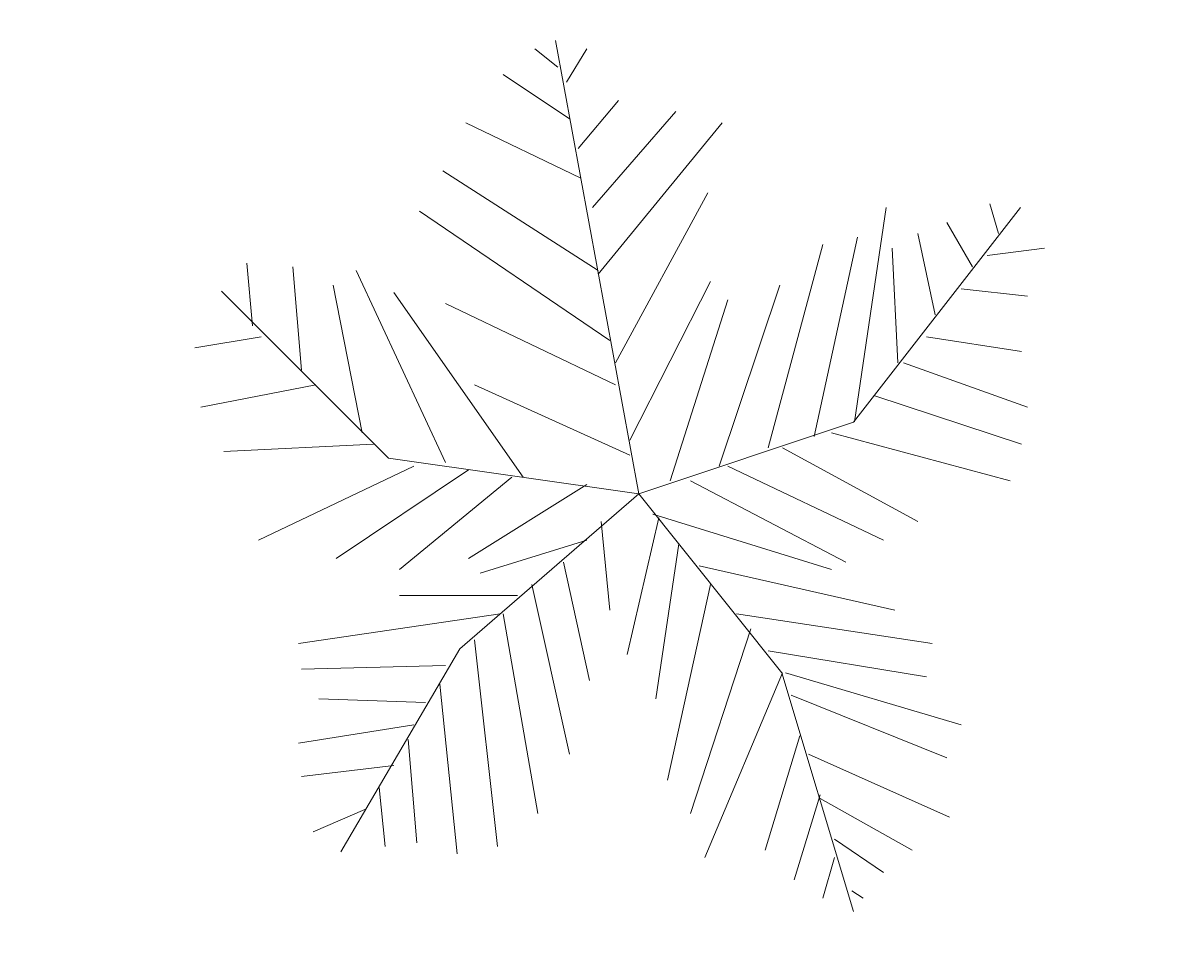
# Model space of a CAD drawing. Units: inches. Extents: x -61 to 1599, y -1316 to 257.
# Tile 127 of 204: x 388 to 418, y -166 to -143. Entities that reach past the tile are written whole.
import ezdxf

# ---------------------------------------------------------------- set-up
doc = ezdxf.new("R2010")
doc.units = ezdxf.units.IN
doc.header["$MEASUREMENT"] = 0
doc.layers.add('A-ANNO-DIMS', color=2, linetype='Continuous', lineweight=18)
doc.layers.add('FURNITURE', color=83, linetype='Continuous', lineweight=18)
doc.styles.get("Standard").update_dxf_attribs({"font": 'arial.ttf'})
doc.dimstyles.get("Standard").update_dxf_attribs({"dimtxt": 0.18, "dimasz": 0.18, "dimexe": 0.18, "dimexo": 0.0625, "dimgap": 0.09, "dimtad": 0, "dimtih": 1, "dimtoh": 1, "dimdec": 0, "dimzin": 0, "dimdsep": 46, "dimlunit": 3, "dimtxsty": 'Standard', "dimcen": 0.09, "dimadec": 0, "dimazin": 0, "dimtfac": 1, "dimtdec": 0, "dimtofl": 0, "dimtmove": 0, "dimatfit": 3, "dimfxl": 1, "dimtolj": 1, "dimtzin": 0, "dimarcsym": 0})

# ---------------------------------------------------------------- blocks, each defined once
blk = doc.blocks.new('*U264')
for p, q in [((0, 0), (-10.5, 57)), ((-10.186, 53.64), (-13.084, 55.962)), ((-9.099, 51.782), (-6.563, 55.962)), ((-8.737, 47.138), (-17.069, 52.711)), ((-7.65, 43.423), (-2.578, 49.46)), ((-5.839, 35.992), (4.667, 48.067)), ((-7.288, 39.707), (-21.778, 46.673)), ((-5.114, 27.632), (10.463, 46.673)), ((-5.114, 28.097), (-24.676, 40.636)), ((-2.941, 16.486), (8.652, 37.85)), ((44.153, 36.456), (45.239, 32.741)), ((-3.665, 19.273), (-27.574, 35.527)), ((27, 9), (48, 36)), ((27.127, 9.056), (31.112, 35.992)), ((38.719, 34.134), (41.979, 28.561)), ((22.055, 7.198), (27.489, 32.277)), ((35.096, 32.741), (37.27, 22.524)), ((16.259, 5.805), (23.142, 31.348)), ((31.836, 30.883), (32.561, 16.486)), ((43.791, 29.954), (51.036, 30.883)), ((-48.585, 21.131), (-49.309, 29.026)), ((-43.513, 28.561), (-42.427, 15.558)), ((-35.544, 28.097), (-24.314, 3.947)), ((-38.442, 26.239), (-34.819, 7.663)), ((-1.129, 6.734), (9.014, 26.704)), ((10.101, 3.483), (17.708, 26.239)), ((-31.5, 4.5), (-52.5, 25.5)), ((-14.533, 2.09), (-30.834, 25.31)), ((40.53, 25.775), (48.862, 24.846)), ((-24.314, 23.917), (-2.941, 13.7)), ((3.942, 1.625), (11.187, 24.381)), ((-47.498, 19.737), (-55.83, 18.344)), ((36.183, 19.737), (48.137, 17.88)), ((33.285, 16.486), (48.862, 10.913)), ((-40.615, 13.7), (-55.105, 10.913)), ((-20.691, 13.7), (-1.129, 4.876)), ((29.662, 12.307), (48.137, 6.269)), ((0, 0), (27, 9)), ((24.229, 7.663), (46.688, 1.625)), ((-33.37, 6.269), (-52.207, 5.34)), ((0, 0), (-31.5, 4.5)), ((18.07, 5.805), (35.096, -3.483)), ((-28.299, 3.483), (-47.86, -5.805)), ((-21.416, 3.018), (-38.079, -8.128)), ((11.187, 3.483), (30.749, -5.805)), ((-15.982, 2.09), (-30.11, -9.521)), ((6.478, 1.625), (26.04, -8.592)), ((0, 0), (-22.5, -19.5)), ((-6.563, 1.161), (-21.416, -8.128)), ((0, 0), (18, -22.5)), ((1.769, -2.555), (24.229, -9.521)), ((-4.752, -3.483), (-3.665, -14.629)), ((2.493, -3.019), (-1.491, -20.202)), ((-6.563, -5.805), (-19.967, -9.985)), ((5.029, -6.27), (2.131, -25.775)), ((-9.461, -8.592), (-6.201, -23.453)), ((7.565, -9.056), (32.198, -14.629)), ((-13.446, -11.378), (-8.737, -32.741)), ((9.014, -11.378), (3.58, -35.992)), ((-15.257, -12.772), (-30.11, -12.772)), ((-17.431, -15.094), (-42.789, -18.809)), ((-17.069, -15.094), (-12.721, -40.172)), ((12.274, -15.094), (36.907, -18.809)), ((14.085, -16.951), (6.478, -40.172)), ((-20.691, -18.345), (-17.793, -44.352)), ((-22.5, -19.5), (-37.5, -45)), ((16.259, -19.738), (36.183, -22.989)), ((-24.314, -21.596), (-42.427, -22.06)), ((18.07, -22.524), (8.289, -45.745)), ((18, -22.5), (27, -52.5)), ((18.433, -22.524), (40.53, -29.026)), ((-25.038, -23.918), (-22.865, -45.281)), ((-26.849, -26.24), (-40.253, -25.775)), ((19.157, -25.311), (38.719, -33.206)), ((-28.299, -29.026), (-42.789, -31.348)), ((20.244, -30.419), (15.897, -44.816)), ((-29.023, -30.884), (-27.936, -43.887)), ((21.331, -32.741), (39.081, -40.636)), ((-30.834, -34.135), (-42.427, -35.528)), ((-32.646, -36.921), (-31.921, -44.352)), ((22.78, -37.85), (19.519, -48.532)), ((22.78, -38.314), (34.372, -44.816)), ((-34.457, -39.708), (-40.978, -42.494)), ((24.591, -43.423), (30.749, -47.603)), ((24.591, -45.745), (23.142, -50.854)), ((26.764, -49.925), (28.213, -50.854))]:
    blk.add_line(p, q)
blk = doc.blocks.new('*D703')
at = {"layer": 'A-ANNO-DIMS', "color": 0, "lineweight": -2, "transparency": 16777216}
for p, q in [((372.32, -616.882), (372.32, 257.457)), ((372.5, 257.277), (413.7, 257.277)), ((455.653, 257.277), (414.453, 257.277)), ((455.833, -616.882), (455.833, 257.457))]:
    blk.add_line(p, q, dxfattribs=at)
at = {"layer": 'A-ANNO-DIMS', "color": 0, "transparency": 16777216}
for points in [[(372.5, 257.307), (372.5, 257.247), (372.32, 257.277)], [(455.653, 257.307), (455.653, 257.247), (455.833, 257.277)]]:
    blk.add_solid(points, dxfattribs=at)
at = {"layer": 'DEFPOINTS', "color": 0, "transparency": 16777216}
for p in [(455.833, 257.277), (372.32, -616.945), (455.833, -616.945)]:
    blk.add_point(p, dxfattribs=at)
at = {"layer": 'A-ANNO-DIMS', "color": 0, "transparency": 16777216, "insert": (414.076, 257.277), "char_height": 0.18, "attachment_point": 5}
blk.add_mtext('\\A1;83.51', dxfattribs=at)

msp = doc.modelspace()

# ---------------------------------------------------------------- block references
at = {"layer": 'FURNITURE', "xscale": 0.2045054661246738, "yscale": 0.2045054661246738, "zscale": 0.2045054661246738}
msp.add_blockref('*U264', (404.3297, -154.712), dxfattribs=at)

# ---------------------------------------------------------------- dimensions: what is measured, and where the dimension line sits
at = {"layer": 'A-ANNO-DIMS'}
dim = msp.add_linear_dim(base=(455.8327, 257.2771), p1=(372.3201, -616.9446), p2=(455.8327, -616.9446), dimstyle='Standard', override={"dimdec": 2, "dimlfac": 1, "dimrnd": 0, "dimzin": 0, "dimdsep": 46, "dimlunit": 2}, dxfattribs=at)
dim.commit()
dim.dimension.update_dxf_attribs({"geometry": '*D703', "text_midpoint": (414.0764, 257.2771)})

doc.saveas('drawing.dxf')
